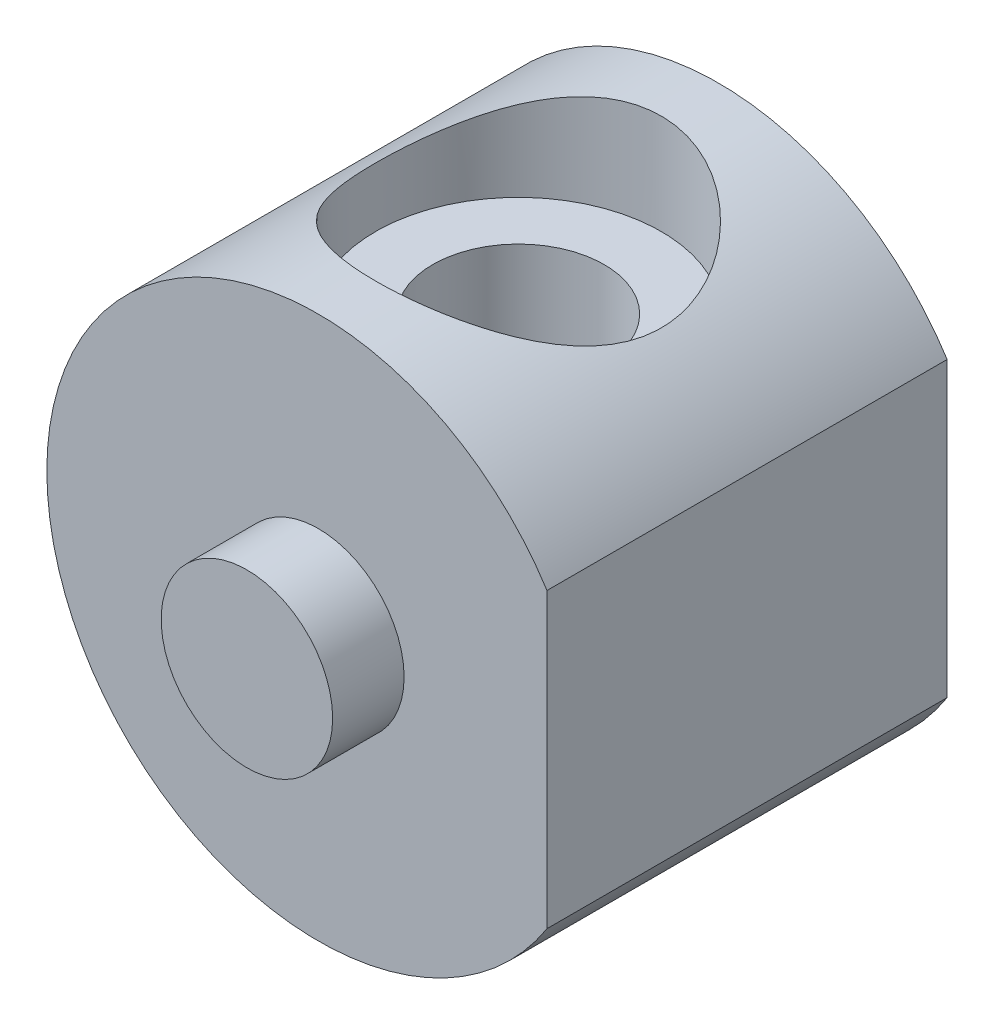
ISO-10303-21;
HEADER;
FILE_DESCRIPTION(('STEP AP214'),'2;1');
FILE_NAME('part.step','',(''),(''),'','','');
FILE_SCHEMA(('AUTOMOTIVE_DESIGN { 1 0 10303 214 1 1 1 1 }'));
ENDSEC;
DATA;
#1=APPLICATION_CONTEXT('core data for automotive mechanical design processes');
#2=APPLICATION_PROTOCOL_DEFINITION('international standard','automotive_design',2000,#1);
#3=PRODUCT_CONTEXT('',#1,'mechanical');
#4=PRODUCT('Part','Part','',(#3));
#5=PRODUCT_RELATED_PRODUCT_CATEGORY('part','',(#4));
#6=PRODUCT_DEFINITION_FORMATION('','',#4);
#7=PRODUCT_DEFINITION_CONTEXT('part definition',#1,'design');
#8=PRODUCT_DEFINITION('design','',#6,#7);
#9=PRODUCT_DEFINITION_SHAPE('','',#8);
#10=(LENGTH_UNIT() NAMED_UNIT(*) SI_UNIT(.MILLI.,.METRE.));
#11=(NAMED_UNIT(*) PLANE_ANGLE_UNIT() SI_UNIT($,.RADIAN.));
#12=(NAMED_UNIT(*) SI_UNIT($,.STERADIAN.) SOLID_ANGLE_UNIT());
#13=UNCERTAINTY_MEASURE_WITH_UNIT(LENGTH_MEASURE(1.E-05),#10,'distance_accuracy_value','');
#14=(GEOMETRIC_REPRESENTATION_CONTEXT(3) GLOBAL_UNCERTAINTY_ASSIGNED_CONTEXT((#13)) GLOBAL_UNIT_ASSIGNED_CONTEXT((#10,
#11,#12)) REPRESENTATION_CONTEXT('',''));
#15=CARTESIAN_POINT('',(0.,0.,0.));
#16=DIRECTION('',(0.,0.,1.));
#17=DIRECTION('',(1.,0.,0.));
#18=AXIS2_PLACEMENT_3D('',#15,#16,#17);
#19=CARTESIAN_POINT('',(0.,0.,14.));
#20=DIRECTION('',(0.,0.,-1.));
#21=DIRECTION('',(-1.,0.,0.));
#22=AXIS2_PLACEMENT_3D('',#19,#20,#21);
#23=CYLINDRICAL_SURFACE('',#22,9.5);
#24=CARTESIAN_POINT('',(0.,-9.5,10.));
#25=CARTESIAN_POINT('',(0.164167089462809,-9.49999935809229,9.9999991920058));
#26=CARTESIAN_POINT('',(0.328342993003654,-9.49570457873447,9.98648026101078));
#27=CARTESIAN_POINT('',(0.651888233262993,-9.47899296182888,9.93290710155364));
#28=CARTESIAN_POINT('',(0.811256566918244,-9.46657444141808,9.89284737504546));
#29=CARTESIAN_POINT('',(1.12047453900869,-9.43497086374047,9.78768208763199));
#30=CARTESIAN_POINT('',(1.2703386681819,-9.4157964146812,9.72261577778607));
#31=CARTESIAN_POINT('',(1.55702915841443,-9.37265725199131,9.56945292714262));
#32=CARTESIAN_POINT('',(1.69385337678599,-9.34869175310374,9.48135261032312));
#33=CARTESIAN_POINT('',(1.954886157509,-9.29766753324294,9.28170532514715));
#34=CARTESIAN_POINT('',(2.07862693177764,-9.27054036694509,9.16956430252643));
#35=CARTESIAN_POINT('',(2.30589485227851,-9.21664353803552,8.92628343975446));
#36=CARTESIAN_POINT('',(2.4094181339002,-9.1898739446838,8.79513997558117));
#37=CARTESIAN_POINT('',(2.59586933707153,-9.1389859370637,8.51350243576824));
#38=CARTESIAN_POINT('',(2.67820924038344,-9.11495183979177,8.36260239311171));
#39=CARTESIAN_POINT('',(2.81614778654471,-9.07328724171044,8.04821507644751));
#40=CARTESIAN_POINT('',(2.87175364335561,-9.05565501372426,7.88473121190931));
#41=CARTESIAN_POINT('',(2.95292728212569,-9.02950721227384,7.55510219526111));
#42=CARTESIAN_POINT('',(2.97936420548708,-9.02072856266505,7.3891925311824));
#43=CARTESIAN_POINT('',(3.00416514791963,-9.01250122204869,7.05507820356029));
#44=CARTESIAN_POINT('',(3.00253681210414,-9.01304999020652,6.8868741774869));
#45=CARTESIAN_POINT('',(2.97193247609429,-9.02318352274045,6.5601689623222));
#46=CARTESIAN_POINT('',(2.94406576248244,-9.03240174793261,6.40155056751834));
#47=CARTESIAN_POINT('',(2.86357596011184,-9.05823941484151,6.0913669451148));
#48=CARTESIAN_POINT('',(2.81095018945963,-9.07485965833217,5.93980248354994));
#49=CARTESIAN_POINT('',(2.68166168169205,-9.11390651918069,5.64540546424869));
#50=CARTESIAN_POINT('',(2.60465367716268,-9.13641567799888,5.50273595369037));
#51=CARTESIAN_POINT('',(2.4290264338323,-9.1846668373259,5.23198235130085));
#52=CARTESIAN_POINT('',(2.33040148183895,-9.21040969170622,5.10390212893102));
#53=CARTESIAN_POINT('',(2.10891443526093,-9.26369376405774,4.859697277003));
#54=CARTESIAN_POINT('',(1.98513792318251,-9.29126291800172,4.74440654185175));
#55=CARTESIAN_POINT('',(1.71966506786238,-9.3440378521759,4.53601351945979));
#56=CARTESIAN_POINT('',(1.57796734157916,-9.36924344974064,4.44291294631118));
#57=CARTESIAN_POINT('',(1.27904248860848,-9.41472566771743,4.28096191105045));
#58=CARTESIAN_POINT('',(1.12169880645912,-9.43496068381886,4.21231410795121));
#59=CARTESIAN_POINT('',(0.796908546050009,-9.46792126212738,4.10271044439606));
#60=CARTESIAN_POINT('',(0.629465120716915,-9.48064915466278,4.06174599002053));
#61=CARTESIAN_POINT('',(0.296303884002125,-9.49678470779038,4.01010108172171));
#62=CARTESIAN_POINT('',(0.130777575905981,-9.50053950796354,3.99829206839531));
#63=CARTESIAN_POINT('',(-0.19991137896084,-9.49933471585785,4.00210623483273));
#64=CARTESIAN_POINT('',(-0.365074076408764,-9.49437642655838,4.01772531292403));
#65=CARTESIAN_POINT('',(-0.68596921290421,-9.47653086922814,4.07504817976814));
#66=CARTESIAN_POINT('',(-0.84183470656139,-9.46384885282509,4.11607718255883));
#67=CARTESIAN_POINT('',(-1.14442314350254,-9.43204434547225,4.22222874627275));
#68=CARTESIAN_POINT('',(-1.29114494807249,-9.41292105424677,4.28735430109444));
#69=CARTESIAN_POINT('',(-1.57531276244697,-9.36960895031318,4.44164618012741));
#70=CARTESIAN_POINT('',(-1.71244019799074,-9.34530669896614,4.53136651414614));
#71=CARTESIAN_POINT('',(-1.97006979650918,-9.29441218727718,4.73163864225214));
#72=CARTESIAN_POINT('',(-2.09056734431474,-9.26781929454284,4.84219619908153));
#73=CARTESIAN_POINT('',(-2.31658675579943,-9.21398298633844,5.08631319348531));
#74=CARTESIAN_POINT('',(-2.42130400734893,-9.186756871098,5.2206231211429));
#75=CARTESIAN_POINT('',(-2.60679013327421,-9.1358594627064,5.50550007708682));
#76=CARTESIAN_POINT('',(-2.68755931108111,-9.11218812451676,5.65606689935918));
#77=CARTESIAN_POINT('',(-2.8223709751743,-9.07133925816319,5.96892389776127));
#78=CARTESIAN_POINT('',(-2.87651039405967,-9.05413823262218,6.13116905384851));
#79=CARTESIAN_POINT('',(-2.95649944180757,-9.0283393693878,6.46312960024526));
#80=CARTESIAN_POINT('',(-2.98236013155669,-9.01973816808891,6.63284204277622));
#81=CARTESIAN_POINT('',(-3.00425241211469,-9.01246833575292,6.96649385186041));
#82=CARTESIAN_POINT('',(-3.00160628169283,-9.01335938768914,7.1303379199969));
#83=CARTESIAN_POINT('',(-2.96976166390158,-9.02390107112083,7.45512331577253));
#84=CARTESIAN_POINT('',(-2.94056446477842,-9.0335512776259,7.61606478385819));
#85=CARTESIAN_POINT('',(-2.8573397985787,-9.06021304876319,7.92805694156504));
#86=CARTESIAN_POINT('',(-2.80369834624608,-9.07710994083738,8.07922114557669));
#87=CARTESIAN_POINT('',(-2.67341300631294,-9.11632984499268,8.3705239915776));
#88=CARTESIAN_POINT('',(-2.59676436934434,-9.13865397723677,8.51066034954493));
#89=CARTESIAN_POINT('',(-2.4190708026092,-9.18732235584319,8.78197349059506));
#90=CARTESIAN_POINT('',(-2.31717569257864,-9.21379131671488,8.91257101653679));
#91=CARTESIAN_POINT('',(-2.0933684813078,-9.26720162412937,9.15524167526138));
#92=CARTESIAN_POINT('',(-1.97145098067163,-9.29414309633804,9.26730979485427));
#93=CARTESIAN_POINT('',(-1.7061326528479,-9.34654886057908,9.47351384861018));
#94=CARTESIAN_POINT('',(-1.56214764703045,-9.37193310874742,9.56692078145933));
#95=CARTESIAN_POINT('',(-1.25971894568572,-9.41734758486009,9.72808336874198));
#96=CARTESIAN_POINT('',(-1.10128066394409,-9.43737980656471,9.79584857926917));
#97=CARTESIAN_POINT('',(-0.78727182995563,-9.468532861615,9.89919753820645));
#98=CARTESIAN_POINT('',(-0.632450266372874,-9.48022921021867,9.93688775917118));
#99=CARTESIAN_POINT('',(-0.318421271901131,-9.49596227615521,9.98728672532889));
#100=CARTESIAN_POINT('',(-0.159214781112169,-9.50000062254375,10.00000078362));
#101=CARTESIAN_POINT('',(0.,-9.5,10.));
#102=B_SPLINE_CURVE_WITH_KNOTS('',3,(#24,#25,#26,#27,#28,#29,#30,#31,#32,#33,#34,#35,#36,#37,
#38,#39,#40,#41,#42,#43,#44,#45,#46,#47,#48,#49,#50,#51,#52,#53,#54,#55,#56,#57,#58,#59,#60,#61,
#62,#63,#64,#65,#66,#67,#68,#69,#70,#71,#72,#73,#74,#75,#76,#77,#78,#79,#80,#81,#82,#83,#84,#85,
#86,#87,#88,#89,#90,#91,#92,#93,#94,#95,#96,#97,#98,#99,#100,#101),.UNSPECIFIED.,.T.,.F.,(4,2,2,
2,2,2,2,2,2,2,2,2,2,2,2,2,2,2,2,2,2,2,2,2,2,2,2,2,2,2,2,2,2,2,2,2,2,2,4),(0.,0.49191594170538,
0.98393381790244,1.47518254201799,1.9665118483056,2.47177433217168,2.97713330355079,
3.49529138086525,4.0133095589189,4.51543663249028,5.01742692636232,5.4991042363361,
5.98083373346493,6.46971527661729,6.95872618352227,7.47049694812961,7.98230723196768,
8.49826565849845,9.01406383907483,9.50955937080917,10.0049808110835,10.487778781206,
10.9706367571643,11.4654198237929,11.9603399289468,12.4753133176055,12.9902801810781,
13.5033584262729,14.0162359151874,14.5054301927743,14.9946007361353,15.4763007218674,
15.9581002132873,16.4590917155026,16.9602185415511,17.4781824310863,17.9959530965539,
18.4731312898967,18.9502079636715),.UNSPECIFIED.);
#103=CARTESIAN_POINT('',(0.,-9.5,10.));
#104=VERTEX_POINT('',#103);
#105=EDGE_CURVE('E47',#104,#104,#102,.T.);
#106=ORIENTED_EDGE('',*,*,#105,.T.);
#107=EDGE_LOOP('',(#106));
#108=FACE_BOUND('',#107,.T.);
#109=CARTESIAN_POINT('',(0.,9.5,12.));
#110=CARTESIAN_POINT('',(-0.130642017435204,9.50000025830867,12.000000317987));
#111=CARTESIAN_POINT('',(-0.261280381095525,9.49729937430302,11.9948744609087));
#112=CARTESIAN_POINT('',(-0.521584051797463,9.48656543983491,11.974434606502));
#113=CARTESIAN_POINT('',(-0.651248987731432,9.47853045078801,11.9591169051265));
#114=CARTESIAN_POINT('',(-0.908724902304482,9.45732130010811,11.9184577717431));
#115=CARTESIAN_POINT('',(-1.03653350028885,9.44414105596159,11.8931044755615));
#116=CARTESIAN_POINT('',(-1.28927680532048,9.41296917939984,11.8326657472864));
#117=CARTESIAN_POINT('',(-1.41421031529785,9.39497558089877,11.7975763381148));
#118=CARTESIAN_POINT('',(-1.65978714859797,9.35470548168469,11.7182284077017));
#119=CARTESIAN_POINT('',(-1.78044717261642,9.33244851287119,11.6740116328295));
#120=CARTESIAN_POINT('',(-2.01738015491985,9.28411689570368,11.5767455040224));
#121=CARTESIAN_POINT('',(-2.13365143738953,9.25804080722284,11.5236928171717));
#122=CARTESIAN_POINT('',(-2.47482405857922,9.17495890241581,11.3520070644262));
#123=CARTESIAN_POINT('',(-2.69233753619866,9.11305607883893,11.2207635075518));
#124=CARTESIAN_POINT('',(-3.11677156857515,8.97711976393962,10.9189251335603));
#125=CARTESIAN_POINT('',(-3.32208711450329,8.90255958431839,10.7463284379279));
#126=CARTESIAN_POINT('',(-3.70237027252013,8.75125016006096,10.3710445731553));
#127=CARTESIAN_POINT('',(-3.87731205508639,8.67449911628705,10.1683320630222));
#128=CARTESIAN_POINT('',(-4.20746485864962,8.51958772864534,9.71698114618832));
#129=CARTESIAN_POINT('',(-4.35957351697895,8.44190043592405,9.46586878456838));
#130=CARTESIAN_POINT('',(-4.55389469941151,8.33771348652021,9.06972121850283));
#131=CARTESIAN_POINT('',(-4.61304200501836,8.30503312029957,8.93437781061485));
#132=CARTESIAN_POINT('',(-4.71942893987689,8.24504198744979,8.65797324544316));
#133=CARTESIAN_POINT('',(-4.76667595821497,8.21772789114389,8.51691569964513));
#134=CARTESIAN_POINT('',(-4.84609400899686,8.1711299546427,8.23893927568855));
#135=CARTESIAN_POINT('',(-4.8790135853186,8.15145552675453,8.10229948531864));
#136=CARTESIAN_POINT('',(-4.93330284979835,8.1187149145794,7.82602781905969));
#137=CARTESIAN_POINT('',(-4.95467900192607,8.10564503220992,7.68639766332513));
#138=CARTESIAN_POINT('',(-4.98553579039544,8.08670284815364,7.40544934672949));
#139=CARTESIAN_POINT('',(-4.99502558557257,8.08082500484111,7.26413257033826));
#140=CARTESIAN_POINT('',(-5.00196707607171,8.0765305257536,6.98109737167334));
#141=CARTESIAN_POINT('',(-4.99942015818057,8.07811303044884,6.83937899754916));
#142=CARTESIAN_POINT('',(-4.9835087363896,8.08793582702385,6.57624055420129));
#143=CARTESIAN_POINT('',(-4.9716676674329,8.09523822735539,6.45468930796877));
#144=CARTESIAN_POINT('',(-4.93920414433694,8.11508625852905,6.21316207725064));
#145=CARTESIAN_POINT('',(-4.91857897557352,8.12763351020944,6.09318659156066));
#146=CARTESIAN_POINT('',(-4.86879569668832,8.15755291872237,5.85564373599223));
#147=CARTESIAN_POINT('',(-4.83963816382844,8.17492474914126,5.73807620377792));
#148=CARTESIAN_POINT('',(-4.77310759932303,8.21394705131997,5.50599946699482));
#149=CARTESIAN_POINT('',(-4.73573131560596,8.23559921641884,5.39149149323216));
#150=CARTESIAN_POINT('',(-4.60993727407042,8.30710221321934,5.04843895868472));
#151=CARTESIAN_POINT('',(-4.5089552304128,8.36280226845538,4.82557825686924));
#152=CARTESIAN_POINT('',(-4.27711316444191,8.48371078685146,4.39896341077218));
#153=CARTESIAN_POINT('',(-4.14623981146092,8.54892348767612,4.19521784866253));
#154=CARTESIAN_POINT('',(-3.83663048089174,8.69272070745621,3.7819125375956));
#155=CARTESIAN_POINT('',(-3.65373132820418,8.77188633784793,3.57566305064235));
#156=CARTESIAN_POINT('',(-3.25568322320281,8.92726591590766,3.19522977888037));
#157=CARTESIAN_POINT('',(-3.04051567525203,9.00347812950142,3.02106461344438));
#158=CARTESIAN_POINT('',(-2.69031313449236,9.11199101243249,2.78292606593711));
#159=CARTESIAN_POINT('',(-2.56527566102103,9.14806544000242,2.70569239191143));
#160=CARTESIAN_POINT('',(-2.30808220172631,9.21631266469039,2.56216106997879));
#161=CARTESIAN_POINT('',(-2.17592927355322,9.24848711868114,2.4958587736205));
#162=CARTESIAN_POINT('',(-1.90541274354747,9.30798472722293,2.3749217991445));
#163=CARTESIAN_POINT('',(-1.76705201224461,9.33531009564093,2.32028179424453));
#164=CARTESIAN_POINT('',(-1.48510653814757,9.38429098896262,2.22332011949645));
#165=CARTESIAN_POINT('',(-1.34152247239194,9.40594724572429,2.18099685953056));
#166=CARTESIAN_POINT('',(-1.06324588010191,9.44126093709507,2.11244534739005));
#167=CARTESIAN_POINT('',(-0.928890040063609,9.45545639827812,2.08512469378947));
#168=CARTESIAN_POINT('',(-0.657922734993127,9.47816515752878,2.0415767075658));
#169=CARTESIAN_POINT('',(-0.521311500568302,9.48667903287943,2.0253482479055));
#170=CARTESIAN_POINT('',(-0.247036826142242,9.49777884344642,2.00421340399773));
#171=CARTESIAN_POINT('',(-0.109373880025652,9.5003674078515,1.99930199812207));
#172=CARTESIAN_POINT('',(0.165866192071598,9.49954860825413,2.00085757220213));
#173=CARTESIAN_POINT('',(0.303443322298543,9.49614156915895,2.00732393558606));
#174=CARTESIAN_POINT('',(0.565238510145971,9.48399374119532,2.03047059473821));
#175=CARTESIAN_POINT('',(0.689565179792539,9.47574957351503,2.04620032997204));
#176=CARTESIAN_POINT('',(0.936335078159328,9.45455545185441,2.08686253871086));
#177=CARTESIAN_POINT('',(1.05877770384544,9.44160402256651,2.11179789739816));
#178=CARTESIAN_POINT('',(1.3009039212563,9.41129768082574,2.17059423676146));
#179=CARTESIAN_POINT('',(1.42058836175402,9.39394414331221,2.20445243063796));
#180=CARTESIAN_POINT('',(1.65653810144973,9.35522364500363,2.28075420602377));
#181=CARTESIAN_POINT('',(1.77280206894129,9.33385514435065,2.32320108203037));
#182=CARTESIAN_POINT('',(2.12128187449469,9.26321206916054,2.46524180583087));
#183=CARTESIAN_POINT('',(2.34711180990764,9.20818884695082,2.57805368478756));
#184=CARTESIAN_POINT('',(2.77719349346286,9.08775319789231,2.83465947491682));
#185=CARTESIAN_POINT('',(2.98143657406127,9.02233662410064,2.97846576104571));
#186=CARTESIAN_POINT('',(3.38565365206916,8.87907718134286,3.31044790692897));
#187=CARTESIAN_POINT('',(3.58289078033236,8.80065182943946,3.50170805126266));
#188=CARTESIAN_POINT('',(3.9439098563227,8.64489981754825,3.91442741905152));
#189=CARTESIAN_POINT('',(4.10766247641555,8.56757417542647,4.13591283486167));
#190=CARTESIAN_POINT('',(4.32972408862321,8.45641507034749,4.49500126326795));
#191=CARTESIAN_POINT('',(4.40152563756837,8.41915698034224,4.62337822295866));
#192=CARTESIAN_POINT('',(4.53389268372542,8.34861864528844,4.88682228881283));
#193=CARTESIAN_POINT('',(4.59446325988689,8.31533660459696,5.02188633570946));
#194=CARTESIAN_POINT('',(4.70366120984529,8.25405932259672,5.29777653864255));
#195=CARTESIAN_POINT('',(4.75229930567555,8.22605934031584,5.43859738810621));
#196=CARTESIAN_POINT('',(4.83702965191852,8.17652491174801,5.72507221017227));
#197=CARTESIAN_POINT('',(4.87312408044718,8.15498934305157,5.87072533886816));
#198=CARTESIAN_POINT('',(4.92928248767462,8.12115384654303,6.15113382693762));
#199=CARTESIAN_POINT('',(4.95056966315995,8.10815628985076,6.28556055118124));
#200=CARTESIAN_POINT('',(4.98212437566265,8.08880605366268,6.55616956106447));
#201=CARTESIAN_POINT('',(4.99239335930639,8.08245250184933,6.69235161386271));
#202=CARTESIAN_POINT('',(5.00174064298667,8.07667140831068,6.96517860928964));
#203=CARTESIAN_POINT('',(5.00082450201333,8.0772404260782,7.1018232882369));
#204=CARTESIAN_POINT('',(4.98783110526358,8.08527049185701,7.37436906711814));
#205=CARTESIAN_POINT('',(4.97575451720252,8.09273112755155,7.51027021104758));
#206=CARTESIAN_POINT('',(4.94268112816605,8.11296668451027,7.76443893864498));
#207=CARTESIAN_POINT('',(4.9228827013437,8.12502408105078,7.88292199255056));
#208=CARTESIAN_POINT('',(4.8749656359116,8.15386310324636,8.11761992670158));
#209=CARTESIAN_POINT('',(4.84684447153816,8.17064616295866,8.2338341069657));
#210=CARTESIAN_POINT('',(4.75042514444156,8.22733743067824,8.57801694456814));
#211=CARTESIAN_POINT('',(4.67005115137982,8.27360072536791,8.8016762481889));
#212=CARTESIAN_POINT('',(4.47370477730413,8.38148159867358,9.2470247968919));
#213=CARTESIAN_POINT('',(4.35574871260941,8.44390522032209,9.46762941778689));
#214=CARTESIAN_POINT('',(4.08956813260782,8.5759838324826,9.88742645472273));
#215=CARTESIAN_POINT('',(3.94132732888993,8.64564270446491,10.0866072597595));
#216=CARTESIAN_POINT('',(3.59465671755025,8.79596127206604,10.4868354003536));
#217=CARTESIAN_POINT('',(3.39210921648311,8.87679892021692,10.6842601145758));
#218=CARTESIAN_POINT('',(2.95476621152202,9.03177925073257,11.0434285524749));
#219=CARTESIAN_POINT('',(2.71995083317694,9.10591775994744,11.2051501245881));
#220=CARTESIAN_POINT('',(2.34500649439869,9.20696916784905,11.4184003306757));
#221=CARTESIAN_POINT('',(2.2147574001187,9.23924127523773,11.4851308248968));
#222=CARTESIAN_POINT('',(1.94804004206673,9.29912751760585,11.6072350656036));
#223=CARTESIAN_POINT('',(1.81157488150005,9.32674394512874,11.6626144045263));
#224=CARTESIAN_POINT('',(1.53368303878259,9.37644427230013,11.7612515491197));
#225=CARTESIAN_POINT('',(1.39226721478332,9.39853950894991,11.8045342156587));
#226=CARTESIAN_POINT('',(1.10544090662377,9.43657275939722,11.8785156219484));
#227=CARTESIAN_POINT('',(0.960032736919906,9.45251426317009,11.9092214949992));
#228=CARTESIAN_POINT('',(0.679250395972509,9.47664083506282,11.955509446457));
#229=CARTESIAN_POINT('',(0.544101109119839,9.48537915156145,11.9721731149942));
#230=CARTESIAN_POINT('',(0.272633236645704,9.49705865313699,11.9944183288481));
#231=CARTESIAN_POINT('',(0.136314629340326,9.4999997304753,11.9999996682057));
#232=CARTESIAN_POINT('',(0.,9.5,12.));
#233=B_SPLINE_CURVE_WITH_KNOTS('',3,(#109,#110,#111,#112,#113,#114,#115,#116,#117,#118,#119,
#120,#121,#122,#123,#124,#125,#126,#127,#128,#129,#130,#131,#132,#133,#134,#135,#136,#137,#138,
#139,#140,#141,#142,#143,#144,#145,#146,#147,#148,#149,#150,#151,#152,#153,#154,#155,#156,#157,
#158,#159,#160,#161,#162,#163,#164,#165,#166,#167,#168,#169,#170,#171,#172,#173,#174,#175,#176,
#177,#178,#179,#180,#181,#182,#183,#184,#185,#186,#187,#188,#189,#190,#191,#192,#193,#194,#195,
#196,#197,#198,#199,#200,#201,#202,#203,#204,#205,#206,#207,#208,#209,#210,#211,#212,#213,#214,
#215,#216,#217,#218,#219,#220,#221,#222,#223,#224,#225,#226,#227,#228,#229,#230,#231,#232),
.UNSPECIFIED.,.T.,.F.,(4,2,2,2,2,2,2,2,2,2,2,2,2,2,2,2,2,2,2,2,2,2,2,2,2,2,2,2,2,2,2,2,2,2,2,2,
2,2,2,2,2,2,2,2,2,2,2,2,2,2,2,2,2,2,2,2,2,2,2,2,2,4),(0.,0.391792234766464,0.783726937376356,
1.17612637938022,1.56868634813667,1.9594891182048,2.35043963476482,3.13153974791819,
3.96336059711627,4.79588538958413,5.70185853857096,6.15514333994223,6.60814599152594,
7.03328551901219,7.4581867336586,7.88276034589864,8.30728504289539,8.67388499400748,
9.04059832088491,9.40728684329944,9.77412072236209,10.5237287019369,11.2736716402267,
12.1305026186323,12.9878292827807,13.4413063432077,13.8945900672075,14.3476663075088,
14.8006840287361,15.2136370748122,15.6265481560021,16.0392759840608,16.4519814467071,
16.8283085214851,17.2047536431578,17.5810813317142,17.9575536488584,18.729187780622,
19.5011305708673,20.3547282709444,21.2090704279473,21.6637716019805,22.1182666436426,
22.5723517866477,23.0263580416498,23.435929262362,23.8454467021029,24.2547606205802,
24.6640500519113,25.0258225662958,25.3877049832792,26.1110184000081,26.8816169531074,
27.6526310629694,28.5313005688989,29.4105137116298,29.8595817113887,30.3084279316799,
30.75634479159,31.2040072492433,31.6128039120318,32.0216081720172),.UNSPECIFIED.);
#234=CARTESIAN_POINT('',(0.,9.5,12.));
#235=VERTEX_POINT('',#234);
#236=EDGE_CURVE('E97',#235,#235,#233,.T.);
#237=ORIENTED_EDGE('',*,*,#236,.T.);
#238=EDGE_LOOP('',(#237));
#239=FACE_BOUND('',#238,.T.);
#240=CARTESIAN_POINT('',(0.,0.,0.));
#241=DIRECTION('',(0.,0.,1.));
#242=DIRECTION('',(1.,0.,0.));
#243=AXIS2_PLACEMENT_3D('',#240,#241,#242);
#244=CIRCLE('',#243,9.5);
#245=CARTESIAN_POINT('',(8.,5.1234753829798,0.));
#246=VERTEX_POINT('',#245);
#247=CARTESIAN_POINT('',(8.,-5.1234753829798,0.));
#248=VERTEX_POINT('',#247);
#249=EDGE_CURVE('E88',#246,#248,#244,.T.);
#250=ORIENTED_EDGE('',*,*,#249,.T.);
#251=DIRECTION('',(0.,0.,-1.));
#252=VECTOR('',#251,1.);
#253=CARTESIAN_POINT('',(8.,-5.1234753829798,14.));
#254=LINE('',#253,#252);
#255=CARTESIAN_POINT('',(8.,-5.1234753829798,14.));
#256=VERTEX_POINT('',#255);
#257=EDGE_CURVE('E81',#256,#248,#254,.T.);
#258=ORIENTED_EDGE('',*,*,#257,.F.);
#259=CARTESIAN_POINT('',(0.,0.,14.));
#260=DIRECTION('',(0.,0.,1.));
#261=DIRECTION('',(1.,0.,0.));
#262=AXIS2_PLACEMENT_3D('',#259,#260,#261);
#263=CIRCLE('',#262,9.5);
#264=CARTESIAN_POINT('',(8.,5.1234753829798,14.));
#265=VERTEX_POINT('',#264);
#266=EDGE_CURVE('E84',#265,#256,#263,.T.);
#267=ORIENTED_EDGE('',*,*,#266,.F.);
#268=DIRECTION('',(0.,0.,-1.));
#269=VECTOR('',#268,1.);
#270=CARTESIAN_POINT('',(8.,5.1234753829798,14.));
#271=LINE('',#270,#269);
#272=EDGE_CURVE('E80',#265,#246,#271,.T.);
#273=ORIENTED_EDGE('',*,*,#272,.T.);
#274=EDGE_LOOP('',(#250,#258,#267,#273));
#275=FACE_BOUND('',#274,.T.);
#276=ADVANCED_FACE('F44',(#108,#239,#275),#23,.T.);
#277=CARTESIAN_POINT('',(8.,5.1234753829798,14.));
#278=DIRECTION('',(-1.,0.,0.));
#279=DIRECTION('',(0.,0.,1.));
#280=AXIS2_PLACEMENT_3D('',#277,#278,#279);
#281=PLANE('',#280);
#282=DIRECTION('',(0.,1.,0.));
#283=VECTOR('',#282,1.);
#284=CARTESIAN_POINT('',(8.,5.1234753829798,0.));
#285=LINE('',#284,#283);
#286=EDGE_CURVE('E73',#248,#246,#285,.T.);
#287=ORIENTED_EDGE('',*,*,#286,.T.);
#288=ORIENTED_EDGE('',*,*,#272,.F.);
#289=DIRECTION('',(0.,1.,0.));
#290=VECTOR('',#289,1.);
#291=CARTESIAN_POINT('',(8.,5.1234753829798,14.));
#292=LINE('',#291,#290);
#293=EDGE_CURVE('E70',#256,#265,#292,.T.);
#294=ORIENTED_EDGE('',*,*,#293,.F.);
#295=ORIENTED_EDGE('',*,*,#257,.T.);
#296=EDGE_LOOP('',(#287,#288,#294,#295));
#297=FACE_BOUND('',#296,.T.);
#298=ADVANCED_FACE('F78',(#297),#281,.F.);
#299=CARTESIAN_POINT('',(0.,0.,14.));
#300=DIRECTION('',(0.,0.,1.));
#301=DIRECTION('',(1.,0.,0.));
#302=AXIS2_PLACEMENT_3D('',#299,#300,#301);
#303=PLANE('',#302);
#304=CARTESIAN_POINT('',(0.,0.,14.));
#305=DIRECTION('',(0.,0.,1.));
#306=DIRECTION('',(1.,0.,0.));
#307=AXIS2_PLACEMENT_3D('',#304,#305,#306);
#308=CIRCLE('',#307,3.);
#309=CARTESIAN_POINT('',(3.,0.,14.));
#310=VERTEX_POINT('',#309);
#311=EDGE_CURVE('E56',#310,#310,#308,.T.);
#312=ORIENTED_EDGE('',*,*,#311,.F.);
#313=EDGE_LOOP('',(#312));
#314=FACE_BOUND('',#313,.T.);
#315=ORIENTED_EDGE('',*,*,#266,.T.);
#316=ORIENTED_EDGE('',*,*,#293,.T.);
#317=EDGE_LOOP('',(#315,#316));
#318=FACE_BOUND('',#317,.T.);
#319=ADVANCED_FACE('F129',(#314,#318),#303,.T.);
#320=CARTESIAN_POINT('',(0.,0.,0.));
#321=DIRECTION('',(0.,0.,1.));
#322=DIRECTION('',(1.,0.,0.));
#323=AXIS2_PLACEMENT_3D('',#320,#321,#322);
#324=PLANE('',#323);
#325=CARTESIAN_POINT('',(0.,0.,0.));
#326=DIRECTION('',(0.,0.,-1.));
#327=DIRECTION('',(-1.,0.,0.));
#328=AXIS2_PLACEMENT_3D('',#325,#326,#327);
#329=CIRCLE('',#328,3.);
#330=CARTESIAN_POINT('',(-3.,0.,0.));
#331=VERTEX_POINT('',#330);
#332=EDGE_CURVE('E11',#331,#331,#329,.T.);
#333=ORIENTED_EDGE('',*,*,#332,.F.);
#334=EDGE_LOOP('',(#333));
#335=FACE_BOUND('',#334,.T.);
#336=ORIENTED_EDGE('',*,*,#249,.F.);
#337=ORIENTED_EDGE('',*,*,#286,.F.);
#338=EDGE_LOOP('',(#336,#337));
#339=FACE_BOUND('',#338,.T.);
#340=ADVANCED_FACE('F89',(#335,#339),#324,.F.);
#341=CARTESIAN_POINT('',(0.,0.,16.5));
#342=DIRECTION('',(0.,0.,-1.));
#343=DIRECTION('',(-1.,0.,0.));
#344=AXIS2_PLACEMENT_3D('',#341,#342,#343);
#345=CYLINDRICAL_SURFACE('',#344,3.);
#346=CARTESIAN_POINT('',(0.,0.,16.5));
#347=DIRECTION('',(0.,0.,1.));
#348=DIRECTION('',(1.,0.,0.));
#349=AXIS2_PLACEMENT_3D('',#346,#347,#348);
#350=CIRCLE('',#349,3.);
#351=CARTESIAN_POINT('',(3.,0.,16.5));
#352=VERTEX_POINT('',#351);
#353=EDGE_CURVE('E93',#352,#352,#350,.T.);
#354=ORIENTED_EDGE('',*,*,#353,.F.);
#355=EDGE_LOOP('',(#354));
#356=FACE_BOUND('',#355,.T.);
#357=ORIENTED_EDGE('',*,*,#311,.T.);
#358=EDGE_LOOP('',(#357));
#359=FACE_BOUND('',#358,.T.);
#360=ADVANCED_FACE('F122',(#356,#359),#345,.T.);
#361=CARTESIAN_POINT('',(0.,0.,16.5));
#362=DIRECTION('',(0.,0.,1.));
#363=DIRECTION('',(1.,0.,0.));
#364=AXIS2_PLACEMENT_3D('',#361,#362,#363);
#365=PLANE('',#364);
#366=ORIENTED_EDGE('',*,*,#353,.T.);
#367=EDGE_LOOP('',(#366));
#368=FACE_BOUND('',#367,.T.);
#369=ADVANCED_FACE('F120',(#368),#365,.T.);
#370=CARTESIAN_POINT('',(0.,0.,-2.5));
#371=DIRECTION('',(0.,0.,1.));
#372=DIRECTION('',(1.,0.,0.));
#373=AXIS2_PLACEMENT_3D('',#370,#371,#372);
#374=CYLINDRICAL_SURFACE('',#373,3.);
#375=CARTESIAN_POINT('',(0.,0.,-2.5));
#376=DIRECTION('',(0.,0.,-1.));
#377=DIRECTION('',(-1.,0.,0.));
#378=AXIS2_PLACEMENT_3D('',#375,#376,#377);
#379=CIRCLE('',#378,3.);
#380=CARTESIAN_POINT('',(-3.,0.,-2.5));
#381=VERTEX_POINT('',#380);
#382=EDGE_CURVE('E94',#381,#381,#379,.T.);
#383=ORIENTED_EDGE('',*,*,#382,.F.);
#384=EDGE_LOOP('',(#383));
#385=FACE_BOUND('',#384,.T.);
#386=ORIENTED_EDGE('',*,*,#332,.T.);
#387=EDGE_LOOP('',(#386));
#388=FACE_BOUND('',#387,.T.);
#389=ADVANCED_FACE('F116',(#385,#388),#374,.T.);
#390=CARTESIAN_POINT('',(0.,0.,-2.5));
#391=DIRECTION('',(0.,0.,-1.));
#392=DIRECTION('',(-1.,0.,0.));
#393=AXIS2_PLACEMENT_3D('',#390,#391,#392);
#394=PLANE('',#393);
#395=ORIENTED_EDGE('',*,*,#382,.T.);
#396=EDGE_LOOP('',(#395));
#397=FACE_BOUND('',#396,.T.);
#398=ADVANCED_FACE('F115',(#397),#394,.T.);
#399=CARTESIAN_POINT('',(0.,6.,7.));
#400=DIRECTION('',(0.,1.,0.));
#401=DIRECTION('',(0.,0.,1.));
#402=AXIS2_PLACEMENT_3D('',#399,#400,#401);
#403=CYLINDRICAL_SURFACE('',#402,5.);
#404=CARTESIAN_POINT('',(0.,6.,7.));
#405=DIRECTION('',(0.,1.,0.));
#406=DIRECTION('',(0.,0.,1.));
#407=AXIS2_PLACEMENT_3D('',#404,#405,#406);
#408=CIRCLE('',#407,5.);
#409=CARTESIAN_POINT('',(0.,6.,12.));
#410=VERTEX_POINT('',#409);
#411=EDGE_CURVE('E104',#410,#410,#408,.T.);
#412=ORIENTED_EDGE('',*,*,#411,.F.);
#413=EDGE_LOOP('',(#412));
#414=FACE_BOUND('',#413,.T.);
#415=ORIENTED_EDGE('',*,*,#236,.F.);
#416=EDGE_LOOP('',(#415));
#417=FACE_BOUND('',#416,.T.);
#418=ADVANCED_FACE('F106',(#414,#417),#403,.F.);
#419=CARTESIAN_POINT('',(0.,6.,7.));
#420=DIRECTION('',(0.,1.,0.));
#421=DIRECTION('',(0.,0.,1.));
#422=AXIS2_PLACEMENT_3D('',#419,#420,#421);
#423=PLANE('',#422);
#424=CARTESIAN_POINT('',(0.,6.,7.));
#425=DIRECTION('',(0.,1.,0.));
#426=DIRECTION('',(0.,0.,1.));
#427=AXIS2_PLACEMENT_3D('',#424,#425,#426);
#428=CIRCLE('',#427,3.);
#429=CARTESIAN_POINT('',(0.,6.,10.));
#430=VERTEX_POINT('',#429);
#431=EDGE_CURVE('E147',#430,#430,#428,.T.);
#432=ORIENTED_EDGE('',*,*,#431,.F.);
#433=EDGE_LOOP('',(#432));
#434=FACE_BOUND('',#433,.T.);
#435=ORIENTED_EDGE('',*,*,#411,.T.);
#436=EDGE_LOOP('',(#435));
#437=FACE_BOUND('',#436,.T.);
#438=ADVANCED_FACE('F112',(#434,#437),#423,.T.);
#439=CARTESIAN_POINT('',(0.,-10.,7.));
#440=DIRECTION('',(0.,1.,0.));
#441=DIRECTION('',(0.,0.,1.));
#442=AXIS2_PLACEMENT_3D('',#439,#440,#441);
#443=CYLINDRICAL_SURFACE('',#442,3.);
#444=ORIENTED_EDGE('',*,*,#431,.T.);
#445=EDGE_LOOP('',(#444));
#446=FACE_BOUND('',#445,.T.);
#447=ORIENTED_EDGE('',*,*,#105,.F.);
#448=EDGE_LOOP('',(#447));
#449=FACE_BOUND('',#448,.T.);
#450=ADVANCED_FACE('F167',(#446,#449),#443,.F.);
#451=CLOSED_SHELL('',(#276,#298,#319,#340,#360,#369,#389,#398,#418,#438,#450));
#452=MANIFOLD_SOLID_BREP('B2',#451);
#453=ADVANCED_BREP_SHAPE_REPRESENTATION('',(#18,#452),#14);
#454=SHAPE_DEFINITION_REPRESENTATION(#9,#453);
ENDSEC;
END-ISO-10303-21;
